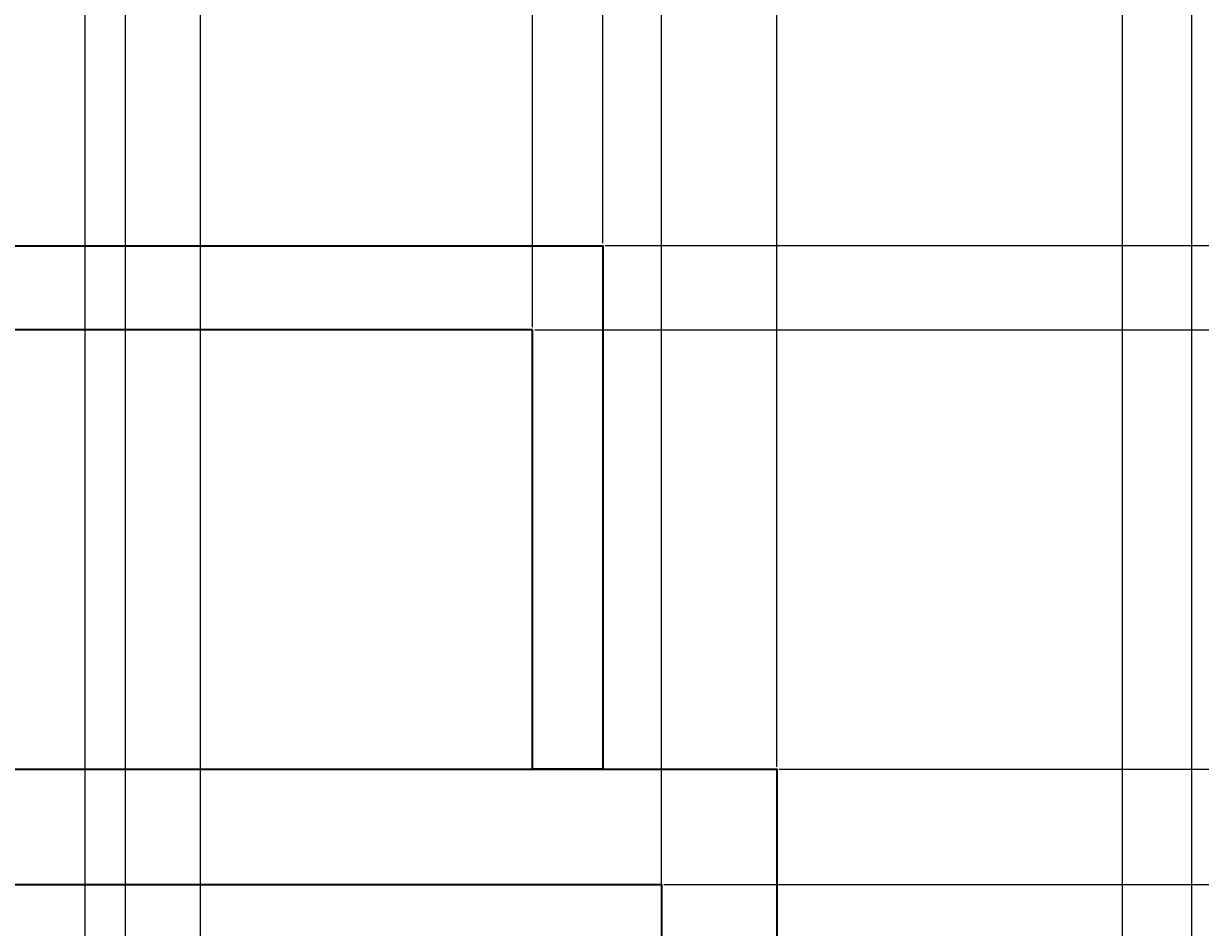
# Model space of a CAD drawing. Units: inches. Extents: x -6 to 289, y -8 to 323.
# Tile 104 of 107: x 243 to 273, y 276 to 299. Entities that reach past the tile are written whole.
import ezdxf

# ---------------------------------------------------------------- set-up
doc = ezdxf.new("R2010")
doc.units = ezdxf.units.IN
doc.header["$MEASUREMENT"] = 0
doc.layers.add('A-ANNO-DIMS', color=2, linetype='Continuous', lineweight=18)
doc.layers.add('A-ELEV', color=7, linetype='Continuous', lineweight=35)
doc.styles.get("Standard").update_dxf_attribs({"font": 'arial.ttf'})
doc.dimstyles.get("Standard").update_dxf_attribs({"dimtxt": 0.18, "dimasz": 0.18, "dimexe": 0.18, "dimexo": 0.0625, "dimgap": 0.09, "dimtad": 0, "dimtih": 1, "dimtoh": 1, "dimdec": 4, "dimzin": 0, "dimdsep": 46, "dimtxsty": 'Standard', "dimcen": 0.09, "dimadec": 0, "dimazin": 0, "dimtfac": 1, "dimtdec": 4, "dimtofl": 0, "dimtmove": 0, "dimatfit": 3, "dimfxl": 1, "dimtolj": 1, "dimtzin": 0, "dimarcsym": 0})

# ---------------------------------------------------------------- blocks, each defined once
blk = doc.blocks.new('*D14')
at = {"layer": 'A-ANNO-DIMS', "color": 0, "lineweight": -2, "transparency": 16777216}
for p, q in [((236.292, 226.951), (236.292, 322.969)), ((247.164, 162.411), (247.164, 322.969)), ((236.472, 322.789), (241.274, 322.789)), ((246.984, 322.789), (242.182, 322.789))]:
    blk.add_line(p, q, dxfattribs=at)
at = {"layer": 'A-ANNO-DIMS', "color": 0, "transparency": 16777216}
for points in [[(236.472, 322.819), (236.472, 322.759), (236.292, 322.789)], [(246.984, 322.819), (246.984, 322.759), (247.164, 322.789)]]:
    blk.add_solid(points, dxfattribs=at)
at = {"layer": 'Defpoints', "color": 0, "transparency": 16777216}
for p in [(247.164, 322.789), (236.292, 226.889), (247.164, 162.348)]:
    blk.add_point(p, dxfattribs=at)
at = {"layer": 'A-ANNO-DIMS', "color": 0, "transparency": 16777216, "insert": (241.728, 322.789), "char_height": 0.18, "attachment_point": 5}
blk.add_mtext('\\A1;10.872', dxfattribs=at)
blk = doc.blocks.new('*D15')
at = {"layer": 'A-ANNO-DIMS', "color": 0, "lineweight": -2, "transparency": 16777216}
for p, q in [((247.164, 162.411), (247.164, 322.969)), ((271.164, 7.351), (271.164, 322.969)), ((247.344, 322.789), (258.944, 322.789)), ((270.984, 322.789), (259.384, 322.789))]:
    blk.add_line(p, q, dxfattribs=at)
at = {"layer": 'A-ANNO-DIMS', "color": 0, "transparency": 16777216}
for points in [[(247.344, 322.819), (247.344, 322.759), (247.164, 322.789)], [(270.984, 322.819), (270.984, 322.759), (271.164, 322.789)]]:
    blk.add_solid(points, dxfattribs=at)
at = {"layer": 'Defpoints', "color": 0, "transparency": 16777216}
for p in [(271.164, 322.789), (247.164, 162.348), (271.164, 7.289)]:
    blk.add_point(p, dxfattribs=at)
at = {"layer": 'A-ANNO-DIMS', "color": 0, "transparency": 16777216, "insert": (259.164, 322.789), "char_height": 0.18, "attachment_point": 5}
blk.add_mtext('\\A1;24', dxfattribs=at)
blk = doc.blocks.new('*D27')
at = {"layer": 'A-ANNO-DIMS', "color": 0, "lineweight": -2, "transparency": 16777216}
for p, q in [((19.226, 307.289), (288.653, 307.289)), ((288.473, 307.109), (288.473, 277.471)), ((288.473, 247.469), (288.473, 277.107)), ((247.226, 247.289), (288.653, 247.289))]:
    blk.add_line(p, q, dxfattribs=at)
at = {"layer": 'A-ANNO-DIMS', "color": 0, "transparency": 16777216}
for points in [[(288.443, 307.109), (288.503, 307.109), (288.473, 307.289)], [(288.443, 247.469), (288.503, 247.469), (288.473, 247.289)]]:
    blk.add_solid(points, dxfattribs=at)
at = {"layer": 'Defpoints', "color": 0, "transparency": 16777216}
for p in [(19.164, 307.289), (288.473, 307.289), (247.164, 247.289)]:
    blk.add_point(p, dxfattribs=at)
at = {"layer": 'A-ANNO-DIMS', "color": 0, "transparency": 16777216, "insert": (288.473, 277.289), "char_height": 0.18, "attachment_point": 5}
blk.add_mtext('\\A1;60', dxfattribs=at)
blk = doc.blocks.new('*D81')
at = {"layer": 'A-ANNO-DIMS', "color": 0, "lineweight": -2, "transparency": 16777216}
for p, q in [((230.292, 68.842), (230.292, 322.969)), ((245.215, 66.286), (245.215, 322.969)), ((230.472, 322.789), (237.298, 322.789)), ((245.035, 322.789), (238.208, 322.789))]:
    blk.add_line(p, q, dxfattribs=at)
at = {"layer": 'A-ANNO-DIMS', "color": 0, "transparency": 16777216}
for points in [[(230.472, 322.819), (230.472, 322.759), (230.292, 322.789)], [(245.035, 322.819), (245.035, 322.759), (245.215, 322.789)]]:
    blk.add_solid(points, dxfattribs=at)
at = {"layer": 'Defpoints', "color": 0, "transparency": 16777216}
for p in [(245.215, 322.789), (230.292, 68.779), (245.215, 66.224)]:
    blk.add_point(p, dxfattribs=at)
at = {"layer": 'A-ANNO-DIMS', "color": 0, "transparency": 16777216, "insert": (237.753, 322.789), "char_height": 0.18, "attachment_point": 5}
blk.add_mtext('\\A1;14.923', dxfattribs=at)
blk = doc.blocks.new('*D82')
at = {"layer": 'A-ANNO-DIMS', "color": 0, "lineweight": -2, "transparency": 16777216}
for p, q in [((245.215, 66.286), (245.215, 322.969)), ((272.973, 66.286), (272.973, 322.969)), ((245.395, 322.789), (258.699, 322.789)), ((272.793, 322.789), (259.489, 322.789))]:
    blk.add_line(p, q, dxfattribs=at)
at = {"layer": 'A-ANNO-DIMS', "color": 0, "transparency": 16777216}
for points in [[(245.395, 322.819), (245.395, 322.759), (245.215, 322.789)], [(272.793, 322.819), (272.793, 322.759), (272.973, 322.789)]]:
    blk.add_solid(points, dxfattribs=at)
at = {"layer": 'Defpoints', "color": 0, "transparency": 16777216}
for p in [(272.973, 322.789), (245.215, 66.224), (272.973, 66.224)]:
    blk.add_point(p, dxfattribs=at)
at = {"layer": 'A-ANNO-DIMS', "color": 0, "transparency": 16777216, "insert": (259.094, 322.789), "char_height": 0.18, "attachment_point": 5}
blk.add_mtext('\\A1;27.76', dxfattribs=at)
blk = doc.blocks.new('*D98')
at = {"layer": 'A-ANNO-DIMS', "color": 0, "lineweight": -2, "transparency": 16777216}
for p, q in [((202.741, 159.411), (202.741, 322.969)), ((244.164, 159.411), (244.164, 322.969)), ((202.921, 322.789), (223.056, 322.789)), ((243.984, 322.789), (223.849, 322.789))]:
    blk.add_line(p, q, dxfattribs=at)
at = {"layer": 'A-ANNO-DIMS', "color": 0, "transparency": 16777216}
for points in [[(202.921, 322.819), (202.921, 322.759), (202.741, 322.789)], [(243.984, 322.819), (243.984, 322.759), (244.164, 322.789)]]:
    blk.add_solid(points, dxfattribs=at)
at = {"layer": 'Defpoints', "color": 0, "transparency": 16777216}
for p in [(244.164, 322.789), (202.741, 159.348), (244.164, 159.348)]:
    blk.add_point(p, dxfattribs=at)
at = {"layer": 'A-ANNO-DIMS', "color": 0, "transparency": 16777216, "insert": (223.452, 322.789), "char_height": 0.18, "attachment_point": 5}
blk.add_mtext('\\A1;41.42', dxfattribs=at)
blk = doc.blocks.new('*D99')
at = {"layer": 'A-ANNO-DIMS', "color": 0, "lineweight": -2, "transparency": 16777216}
for p, q in [((244.164, 159.411), (244.164, 322.969)), ((247.164, 162.411), (247.164, 322.969)), ((244.344, 322.789), (245.515, 322.789)), ((246.984, 322.789), (245.813, 322.789))]:
    blk.add_line(p, q, dxfattribs=at)
at = {"layer": 'A-ANNO-DIMS', "color": 0, "transparency": 16777216}
for points in [[(244.344, 322.819), (244.344, 322.759), (244.164, 322.789)], [(246.984, 322.819), (246.984, 322.759), (247.164, 322.789)]]:
    blk.add_solid(points, dxfattribs=at)
at = {"layer": 'Defpoints', "color": 0, "transparency": 16777216}
for p in [(247.164, 322.789), (247.164, 162.348), (244.164, 159.348)]:
    blk.add_point(p, dxfattribs=at)
at = {"layer": 'A-ANNO-DIMS', "color": 0, "transparency": 16777216, "insert": (245.664, 322.789), "char_height": 0.18, "attachment_point": 5}
blk.add_mtext('\\A1;3', dxfattribs=at)
blk = doc.blocks.new('*D100')
at = {"layer": 'A-ANNO-DIMS', "color": 0, "lineweight": -2, "transparency": 16777216}
for p, q in [((247.164, 162.411), (247.164, 322.969)), ((259.164, 139.351), (259.164, 322.969)), ((247.344, 322.789), (252.954, 322.789)), ((258.984, 322.789), (253.373, 322.789))]:
    blk.add_line(p, q, dxfattribs=at)
at = {"layer": 'A-ANNO-DIMS', "color": 0, "transparency": 16777216}
for points in [[(247.344, 322.819), (247.344, 322.759), (247.164, 322.789)], [(258.984, 322.819), (258.984, 322.759), (259.164, 322.789)]]:
    blk.add_solid(points, dxfattribs=at)
at = {"layer": 'Defpoints', "color": 0, "transparency": 16777216}
for p in [(259.164, 322.789), (247.164, 162.348), (259.164, 139.289)]:
    blk.add_point(p, dxfattribs=at)
at = {"layer": 'A-ANNO-DIMS', "color": 0, "transparency": 16777216, "insert": (253.164, 322.789), "char_height": 0.18, "attachment_point": 5}
blk.add_mtext('\\A1;12', dxfattribs=at)
blk = doc.blocks.new('*D108')
at = {"layer": 'A-ANNO-DIMS', "color": 0, "lineweight": -2, "transparency": 16777216}
for p, q in [((186.984, 291.541), (186.984, 322.969)), ((255.804, 291.541), (255.804, 322.969)), ((187.164, 322.789), (221, 322.789)), ((255.624, 322.789), (221.787, 322.789))]:
    blk.add_line(p, q, dxfattribs=at)
at = {"layer": 'A-ANNO-DIMS', "color": 0, "transparency": 16777216}
for points in [[(187.164, 322.819), (187.164, 322.759), (186.984, 322.789)], [(255.624, 322.819), (255.624, 322.759), (255.804, 322.789)]]:
    blk.add_solid(points, dxfattribs=at)
at = {"layer": 'Defpoints', "color": 0, "transparency": 16777216}
for p in [(255.804, 322.789), (186.984, 291.478), (255.804, 291.478)]:
    blk.add_point(p, dxfattribs=at)
at = {"layer": 'A-ANNO-DIMS', "color": 0, "transparency": 16777216, "insert": (221.394, 322.789), "char_height": 0.18, "attachment_point": 5}
blk.add_mtext('\\A1;68.82', dxfattribs=at)
blk = doc.blocks.new('*D109')
at = {"layer": 'A-ANNO-DIMS', "color": 0, "lineweight": -2, "transparency": 16777216}
for p, q in [((255.804, 291.541), (255.804, 322.969)), ((257.641, 293.728), (257.641, 322.969)), ((255.984, 322.789), (256.337, 322.789)), ((257.461, 322.789), (257.107, 322.789))]:
    blk.add_line(p, q, dxfattribs=at)
at = {"layer": 'A-ANNO-DIMS', "color": 0, "transparency": 16777216}
for points in [[(255.984, 322.819), (255.984, 322.759), (255.804, 322.789)], [(257.461, 322.819), (257.461, 322.759), (257.641, 322.789)]]:
    blk.add_solid(points, dxfattribs=at)
at = {"layer": 'Defpoints', "color": 0, "transparency": 16777216}
for p in [(257.641, 322.789), (257.641, 293.666), (255.804, 291.478)]:
    blk.add_point(p, dxfattribs=at)
at = {"layer": 'A-ANNO-DIMS', "color": 0, "transparency": 16777216, "insert": (256.722, 322.789), "char_height": 0.18, "attachment_point": 5}
blk.add_mtext('\\A1;1.837', dxfattribs=at)
blk = doc.blocks.new('*D110')
at = {"layer": 'A-ANNO-DIMS', "color": 0, "lineweight": -2, "transparency": 16777216}
for p, q in [((257.641, 293.728), (257.641, 322.969)), ((259.164, 277.105), (259.164, 322.969)), ((257.821, 322.789), (258.017, 322.789)), ((258.984, 322.789), (258.787, 322.789))]:
    blk.add_line(p, q, dxfattribs=at)
at = {"layer": 'A-ANNO-DIMS', "color": 0, "transparency": 16777216}
for points in [[(257.821, 322.819), (257.821, 322.759), (257.641, 322.789)], [(258.984, 322.819), (258.984, 322.759), (259.164, 322.789)]]:
    blk.add_solid(points, dxfattribs=at)
at = {"layer": 'Defpoints', "color": 0, "transparency": 16777216}
for p in [(259.164, 322.789), (257.641, 293.666), (259.164, 277.043)]:
    blk.add_point(p, dxfattribs=at)
at = {"layer": 'A-ANNO-DIMS', "color": 0, "transparency": 16777216, "insert": (258.402, 322.789), "char_height": 0.18, "attachment_point": 5}
blk.add_mtext('\\A1;1.523', dxfattribs=at)
blk = doc.blocks.new('*D111')
at = {"layer": 'A-ANNO-DIMS', "color": 0, "lineweight": -2, "transparency": 16777216}
for p, q in [((259.164, 277.105), (259.164, 322.969)), ((262.164, 280.105), (262.164, 322.969)), ((259.344, 322.789), (260.515, 322.789)), ((261.984, 322.789), (260.813, 322.789))]:
    blk.add_line(p, q, dxfattribs=at)
at = {"layer": 'A-ANNO-DIMS', "color": 0, "transparency": 16777216}
for points in [[(259.344, 322.819), (259.344, 322.759), (259.164, 322.789)], [(261.984, 322.819), (261.984, 322.759), (262.164, 322.789)]]:
    blk.add_solid(points, dxfattribs=at)
at = {"layer": 'Defpoints', "color": 0, "transparency": 16777216}
for p in [(262.164, 322.789), (262.164, 280.043), (259.164, 277.043)]:
    blk.add_point(p, dxfattribs=at)
at = {"layer": 'A-ANNO-DIMS', "color": 0, "transparency": 16777216, "insert": (260.664, 322.789), "char_height": 0.18, "attachment_point": 5}
blk.add_mtext('\\A1;3', dxfattribs=at)
blk = doc.blocks.new('*D112')
at = {"layer": 'A-ANNO-DIMS', "color": 0, "lineweight": -2, "transparency": 16777216}
for p, q in [((262.164, 280.105), (262.164, 322.969)), ((271.164, 259.351), (271.164, 322.969)), ((262.344, 322.789), (266.515, 322.789)), ((270.984, 322.789), (266.813, 322.789))]:
    blk.add_line(p, q, dxfattribs=at)
at = {"layer": 'A-ANNO-DIMS', "color": 0, "transparency": 16777216}
for points in [[(262.344, 322.819), (262.344, 322.759), (262.164, 322.789)], [(270.984, 322.819), (270.984, 322.759), (271.164, 322.789)]]:
    blk.add_solid(points, dxfattribs=at)
at = {"layer": 'Defpoints', "color": 0, "transparency": 16777216}
for p in [(271.164, 322.789), (262.164, 280.043), (271.164, 259.289)]:
    blk.add_point(p, dxfattribs=at)
at = {"layer": 'A-ANNO-DIMS', "color": 0, "transparency": 16777216, "insert": (266.664, 322.789), "char_height": 0.18, "attachment_point": 5}
blk.add_mtext('\\A1;9', dxfattribs=at)
blk = doc.blocks.new('*D114')
at = {"layer": 'A-ANNO-DIMS', "color": 0, "lineweight": -2, "transparency": 16777216}
for p, q in [((259.226, 277.043), (288.653, 277.043)), ((288.473, 276.863), (288.473, 268.348)), ((288.473, 259.469), (288.473, 267.984)), ((271.226, 259.289), (288.653, 259.289))]:
    blk.add_line(p, q, dxfattribs=at)
at = {"layer": 'A-ANNO-DIMS', "color": 0, "transparency": 16777216}
for points in [[(288.443, 276.863), (288.503, 276.863), (288.473, 277.043)], [(288.443, 259.469), (288.503, 259.469), (288.473, 259.289)]]:
    blk.add_solid(points, dxfattribs=at)
at = {"layer": 'Defpoints', "color": 0, "transparency": 16777216}
for p in [(259.164, 277.043), (288.473, 277.043), (271.164, 259.289)]:
    blk.add_point(p, dxfattribs=at)
at = {"layer": 'A-ANNO-DIMS', "color": 0, "transparency": 16777216, "insert": (288.473, 268.166), "char_height": 0.18, "attachment_point": 5}
blk.add_mtext('\\A1;17.754', dxfattribs=at)
blk = doc.blocks.new('*D115')
at = {"layer": 'A-ANNO-DIMS', "color": 0, "lineweight": -2, "transparency": 16777216}
for p, q in [((262.226, 280.043), (288.653, 280.043)), ((288.473, 279.863), (288.473, 278.725)), ((288.473, 277.223), (288.473, 278.361)), ((259.226, 277.043), (288.653, 277.043))]:
    blk.add_line(p, q, dxfattribs=at)
at = {"layer": 'A-ANNO-DIMS', "color": 0, "transparency": 16777216}
for points in [[(288.443, 279.863), (288.503, 279.863), (288.473, 280.043)], [(288.443, 277.223), (288.503, 277.223), (288.473, 277.043)]]:
    blk.add_solid(points, dxfattribs=at)
at = {"layer": 'Defpoints', "color": 0, "transparency": 16777216}
for p in [(262.164, 280.043), (288.473, 280.043), (259.164, 277.043)]:
    blk.add_point(p, dxfattribs=at)
at = {"layer": 'A-ANNO-DIMS', "color": 0, "transparency": 16777216, "insert": (288.473, 278.543), "char_height": 0.18, "attachment_point": 5}
blk.add_mtext('\\A1;3', dxfattribs=at)
blk = doc.blocks.new('*D116')
at = {"layer": 'A-ANNO-DIMS', "color": 0, "lineweight": -2, "transparency": 16777216}
for p, q in [((255.866, 291.478), (288.653, 291.478)), ((288.473, 291.298), (288.473, 285.942)), ((288.473, 280.223), (288.473, 285.578)), ((262.226, 280.043), (288.653, 280.043))]:
    blk.add_line(p, q, dxfattribs=at)
at = {"layer": 'A-ANNO-DIMS', "color": 0, "transparency": 16777216}
for points in [[(288.443, 291.298), (288.503, 291.298), (288.473, 291.478)], [(288.443, 280.223), (288.503, 280.223), (288.473, 280.043)]]:
    blk.add_solid(points, dxfattribs=at)
at = {"layer": 'Defpoints', "color": 0, "transparency": 16777216}
for p in [(255.804, 291.478), (288.473, 291.478), (262.164, 280.043)]:
    blk.add_point(p, dxfattribs=at)
at = {"layer": 'A-ANNO-DIMS', "color": 0, "transparency": 16777216, "insert": (288.473, 285.76), "char_height": 0.18, "attachment_point": 5}
blk.add_mtext('\\A1;11.435', dxfattribs=at)
blk = doc.blocks.new('*D117')
at = {"layer": 'A-ANNO-DIMS', "color": 0, "lineweight": -2, "transparency": 16777216}
for p, q in [((257.703, 293.666), (288.653, 293.666)), ((288.473, 293.486), (288.473, 292.754)), ((288.473, 291.658), (288.473, 292.39)), ((255.866, 291.478), (288.653, 291.478))]:
    blk.add_line(p, q, dxfattribs=at)
at = {"layer": 'A-ANNO-DIMS', "color": 0, "transparency": 16777216}
for points in [[(288.443, 293.486), (288.503, 293.486), (288.473, 293.666)], [(288.443, 291.658), (288.503, 291.658), (288.473, 291.478)]]:
    blk.add_solid(points, dxfattribs=at)
at = {"layer": 'Defpoints', "color": 0, "transparency": 16777216}
for p in [(257.641, 293.666), (288.473, 293.666), (255.804, 291.478)]:
    blk.add_point(p, dxfattribs=at)
at = {"layer": 'A-ANNO-DIMS', "color": 0, "transparency": 16777216, "insert": (288.473, 292.572), "char_height": 0.18, "attachment_point": 5}
blk.add_mtext('\\A1;2.19', dxfattribs=at)
blk = doc.blocks.new('*D118')
at = {"layer": 'A-ANNO-DIMS', "color": 0, "lineweight": -2, "transparency": 16777216}
for p, q in [((118.226, 307.289), (288.653, 307.289)), ((288.473, 307.109), (288.473, 300.659)), ((288.473, 293.846), (288.473, 300.295)), ((257.703, 293.666), (288.653, 293.666))]:
    blk.add_line(p, q, dxfattribs=at)
at = {"layer": 'A-ANNO-DIMS', "color": 0, "transparency": 16777216}
for points in [[(288.443, 307.109), (288.503, 307.109), (288.473, 307.289)], [(288.443, 293.846), (288.503, 293.846), (288.473, 293.666)]]:
    blk.add_solid(points, dxfattribs=at)
at = {"layer": 'Defpoints', "color": 0, "transparency": 16777216}
for p in [(118.164, 307.289), (288.473, 307.289), (257.641, 293.666)]:
    blk.add_point(p, dxfattribs=at)
at = {"layer": 'A-ANNO-DIMS', "color": 0, "transparency": 16777216, "insert": (288.473, 300.477), "char_height": 0.18, "attachment_point": 5}
blk.add_mtext('\\A1;13.623', dxfattribs=at)

msp = doc.modelspace()

# ---------------------------------------------------------------- linework, layer by layer
at = {"layer": 'A-ELEV'}
for points in [[(115.1638, 307.2888), (115.1638, 277.0427), (259.1638, 277.0427), (259.1638, 259.2888)], [(118.1638, 307.2888), (118.1638, 280.0427), (262.1638, 280.0427), (262.1638, 259.2888)], [(255.8036, 291.4781), (118.1638, 291.4781), (118.1638, 293.6657), (255.8036, 293.6657)], [(255.8036, 293.6657), (257.6407, 293.6657), (257.6407, 280.0427), (255.8036, 280.0427), (255.8036, 291.4781)]]:
    msp.add_lwpolyline(points, dxfattribs=at)

# ---------------------------------------------------------------- dimensions: what is measured, and where the dimension line sits
at = {"layer": 'A-ANNO-DIMS'}
for base, p1, p2, override, picture, middle in [((255.8036, 322.7888), (186.9837, 291.4781), (255.8036, 291.4781), {"dimdec": 2, "dimlfac": 1, "dimrnd": 0, "dimzin": 0, "dimdsep": 46, "dimlunit": 2}, '*D108', (221.3936, 322.7888)), ((244.1638, 322.7888), (202.741, 159.3484), (244.1638, 159.3484), {"dimdec": 2, "dimlfac": 1, "dimrnd": 0, "dimzin": 0, "dimdsep": 46, "dimlunit": 2}, '*D98', (223.4524, 322.7888)), ((245.2146, 322.7888), (230.2918, 68.7795), (245.2146, 66.2238), {"dimdec": 3, "dimlfac": 1, "dimrnd": 0, "dimzin": 0, "dimdsep": 46, "dimlunit": 2}, '*D81', (237.7532, 322.7888)), ((247.1638, 322.7888), (236.2918, 226.8887), (247.1638, 162.3484), {"dimdec": 3, "dimlfac": 1, "dimrnd": 0, "dimzin": 0, "dimdsep": 46, "dimlunit": 2}, '*D14', (241.7278, 322.7888)), ((247.1638, 322.7888), (244.1638, 159.3484), (247.1638, 162.3484), {"dimdec": 0, "dimlfac": 1, "dimrnd": 0, "dimzin": 0, "dimdsep": 46, "dimlunit": 2}, '*D99', (245.6638, 322.7888)), ((272.9733, 322.7888), (245.2146, 66.2238), (272.9733, 66.2238), {"dimdec": 2, "dimlfac": 1, "dimrnd": 0, "dimzin": 0, "dimdsep": 46, "dimlunit": 2}, '*D82', (259.0939, 322.7888)), ((271.1638, 322.7888), (247.1638, 162.3484), (271.1638, 7.2888), {"dimdec": 0, "dimlfac": 1, "dimrnd": 0, "dimzin": 0, "dimdsep": 46, "dimlunit": 2}, '*D15', (259.1638, 322.7888)), ((259.1638, 322.7888), (247.1638, 162.3484), (259.1638, 139.2888), {"dimdec": 0, "dimlfac": 1, "dimrnd": 0, "dimzin": 0, "dimdsep": 46, "dimlunit": 2}, '*D100', (253.1638, 322.7888)), ((257.6407, 322.7888), (255.8036, 291.4781), (257.6407, 293.6657), {"dimdec": 3, "dimlfac": 1, "dimrnd": 0, "dimzin": 0, "dimdsep": 46, "dimlunit": 2}, '*D109', (256.7221, 322.7888)), ((259.1638, 322.7888), (257.6407, 293.6657), (259.1638, 277.0427), {"dimdec": 3, "dimlfac": 1, "dimrnd": 0, "dimzin": 0, "dimdsep": 46, "dimlunit": 2}, '*D110', (258.4022, 322.7888)), ((262.1638, 322.7888), (259.1638, 277.0427), (262.1638, 280.0427), {"dimdec": 0, "dimlfac": 1, "dimrnd": 0, "dimzin": 0, "dimdsep": 46, "dimlunit": 2}, '*D111', (260.6638, 322.7888)), ((271.1638, 322.7888), (262.1638, 280.0427), (271.1638, 259.2888), {"dimdec": 0, "dimlfac": 1, "dimrnd": 0, "dimzin": 0, "dimdsep": 46, "dimlunit": 2}, '*D112', (266.6638, 322.7888))]:
    dim = msp.add_linear_dim(base=base, p1=p1, p2=p2, dimstyle='Standard', override=override, dxfattribs=at)
    dim.commit()
    dim.dimension.update_dxf_attribs({"geometry": picture, "text_midpoint": middle})
for base, p1, p2, override, picture, middle in [((288.4733, 307.2888), (247.1638, 247.2888), (19.1638, 307.2888), {"dimdec": 0, "dimlfac": 1, "dimrnd": 0, "dimzin": 0, "dimdsep": 46, "dimlunit": 2}, '*D27', (288.4733, 277.2888)), ((288.4733, 307.2888), (257.6407, 293.6657), (118.1638, 307.2888), {"dimdec": 3, "dimlfac": 1, "dimrnd": 0, "dimzin": 0, "dimdsep": 46, "dimlunit": 2}, '*D118', (288.4733, 300.4773)), ((288.4733, 293.6657), (255.8036, 291.4781), (257.6407, 293.6657), {"dimdec": 2, "dimlfac": 1, "dimrnd": 0, "dimzin": 0, "dimdsep": 46, "dimlunit": 2}, '*D117', (288.4733, 292.5719)), ((288.4733, 291.4781), (262.1638, 280.0427), (255.8036, 291.4781), {"dimdec": 3, "dimlfac": 1, "dimrnd": 0, "dimzin": 0, "dimdsep": 46, "dimlunit": 2}, '*D116', (288.4733, 285.7604)), ((288.4733, 280.0427), (259.1638, 277.0427), (262.1638, 280.0427), {"dimdec": 0, "dimlfac": 1, "dimrnd": 0, "dimzin": 0, "dimdsep": 46, "dimlunit": 2}, '*D115', (288.4733, 278.5427)), ((288.4733, 277.0427), (271.1638, 259.2888), (259.1638, 277.0427), {"dimdec": 3, "dimlfac": 1, "dimrnd": 0, "dimzin": 0, "dimdsep": 46, "dimlunit": 2}, '*D114', (288.4733, 268.1657))]:
    dim = msp.add_linear_dim(base=base, p1=p1, p2=p2, angle=90, dimstyle='Standard', override=override, dxfattribs=at)
    dim.commit()
    dim.dimension.update_dxf_attribs({"geometry": picture, "text_midpoint": middle})

doc.saveas('drawing.dxf')
